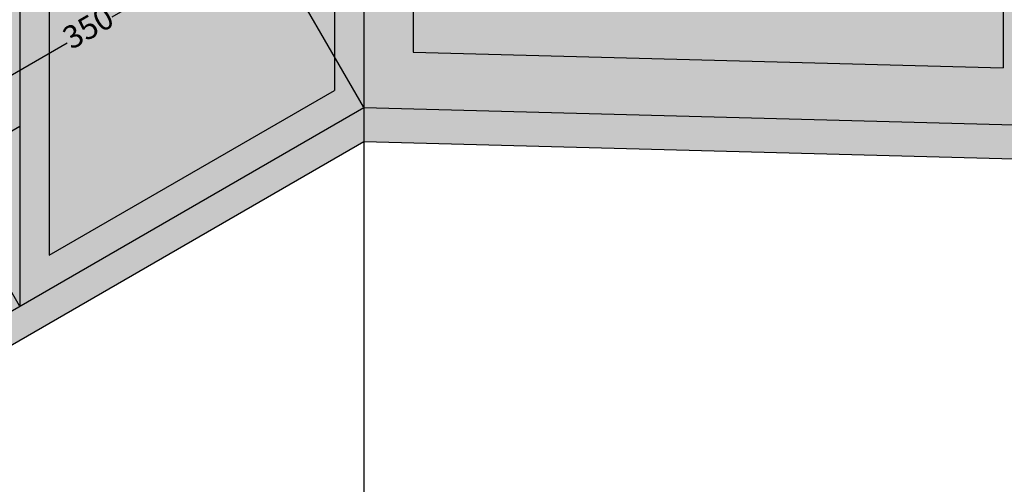
# Model space of a CAD drawing. Units: millimetres. Extents: x 78378 to 86415, y 148682 to 152721.
# Tile 7 of 18: x 79783 to 80650, y 149298 to 149707. Entities that reach past the tile are written whole.
import ezdxf

# ---------------------------------------------------------------- set-up
doc = ezdxf.new("R2010")
doc.units = ezdxf.units.MM
for name, color, linetype, lineweight in [('A-ANNO-DIMS', 2, 'Continuous', 18), ('A-FURN', 4, 'Continuous', 25), ('A-FURN-PATT', 32, 'Continuous', 13)]:
    doc.layers.add(name, color=color, linetype=linetype, lineweight=lineweight)
doc.styles.get("Standard").update_dxf_attribs({"font": 'arial.ttf'})
doc.dimstyles.new('ISO-25', dxfattribs={"dimtxt": 20, "dimasz": 20, "dimexe": 1.25, "dimexo": 0.625, "dimtad": 0, "dimdec": 1, "dimtxsty": 'Standard', "dimcen": 2.5, "dimadec": 0, "dimazin": 0, "dimtfac": 1, "dimtdec": 1, "dimtmove": 0, "dimatfit": 3, "dimfxl": 1, "dimarcsym": 0})

# ---------------------------------------------------------------- blocks, each defined once
blk = doc.blocks.new('*D22')
at = {"layer": 'A-ANNO-DIMS', "color": 0, "lineweight": -2, "transparency": 16777216}
for p, q in [((80086.09, 149630.55), (79995.78, 149786.97)), ((79979.08, 149775.89), (79864.49, 149709.73)), ((79710.62, 149620.89), (79825.21, 149687.05)), ((79782.98, 149455.55), (79692.67, 149611.97))]:
    blk.add_line(p, q, dxfattribs=at)
at = {"layer": 'A-ANNO-DIMS', "color": 0, "transparency": 16777216}
for points in [[(79977.42, 149778.78), (79980.75, 149773.01), (79996.4, 149785.89)], [(79708.95, 149623.78), (79712.28, 149618.01), (79693.3, 149610.89)]]:
    blk.add_solid(points, dxfattribs=at)
at = {"layer": 'Defpoints', "color": 0, "transparency": 16777216}
for p in [(79996.4, 149785.89), (80086.4, 149630.01), (79783.3, 149455.01)]:
    blk.add_point(p, dxfattribs=at)
at = {"layer": 'A-ANNO-DIMS', "color": 0, "transparency": 16777216, "insert": (79844.85, 149698.39), "char_height": 20, "attachment_point": 5, "rotation": 30}
blk.add_mtext('350', dxfattribs=at)
blk = doc.blocks.new('*D32')
at = {"layer": 'A-ANNO-DIMS', "color": 0, "lineweight": -2, "transparency": 16777216}
for p, q in [((80086.4, 150459.38), (80086.4, 148693.76)), ((80692.62, 150459.38), (80692.62, 148693.76)), ((80106.4, 148695.01), (80355.19, 148695.01)), ((80672.62, 148695.01), (80423.84, 148695.01))]:
    blk.add_line(p, q, dxfattribs=at)
at = {"layer": 'A-ANNO-DIMS', "color": 0, "transparency": 16777216}
for points in [[(80106.4, 148698.34), (80106.4, 148691.67), (80086.4, 148695.01)], [(80672.62, 148698.34), (80672.62, 148691.67), (80692.62, 148695.01)]]:
    blk.add_solid(points, dxfattribs=at)
at = {"layer": 'Defpoints', "color": 0, "transparency": 16777216}
for p in [(80086.4, 150460.01), (80692.62, 150460.01), (80692.62, 148695.01)]:
    blk.add_point(p, dxfattribs=at)
at = {"layer": 'A-ANNO-DIMS', "color": 0, "transparency": 16777216, "insert": (80389.51, 148695.01), "char_height": 20, "attachment_point": 5}
blk.add_mtext('606.2', dxfattribs=at)

msp = doc.modelspace()

# ---------------------------------------------------------------- hatches: boundary and pattern name
at = {"layer": 'A-FURN-PATT'}
h = msp.add_hatch(color=256, dxfattribs=at)
h.dxf.hatch_style = 1
h.paths.add_polyline_path([(80692.622, 150440.0076), (80086.4042, 150440.0076), (80086.4042, 149630.0076), (80692.622, 149614.0076)])
h.paths.add_polyline_path([(80293.421, 150335.1041, -0.69391375), (80505.0284, 150344.716, -0.266338), (80649.3207, 150178.1039), (80649.3207, 149665.1505), (80129.7055, 149678.8648), (80129.7055, 150178.1039, -0.25732621)], flags=16)
h.paths.add_polyline_path([(80060.4234, 150384.3024), (79809.2761, 150239.3024), (79809.2761, 150141.6366), (80060.4234, 150286.6366)])
h.paths.add_polyline_path([(80086.4042, 150399.3024), (80086.4042, 150440.0076), (79783.2953, 150265.0076), (79783.2953, 150224.3024)])
edge = h.paths.add_edge_path(flags=16)
edge.add_arc((79946.6302, 150348.8763), 10.7636, -18.3817969, 28.0331994, ccw=False)
edge.add_spline(control_points=[(79956.8447, 150345.482), (79949.4862, 150336.2391), (79933.8528, 150316.6023), (79908.9507, 150312.562), (79895.7699, 150310.4234)], knot_values=[0, 0, 0, 0, 34.22568399, 72.71357657, 72.71357657, 72.71357657, 72.71357657], degree=3, periodic=0)
edge.add_arc((79899.3869, 150314.0155), 5.0977, 123.6496153, 224.8024751, ccw=False)
edge.add_spline(control_points=[(79896.5622, 150318.259), (79909.861, 150320.2803), (79934.7821, 150324.0679), (79949.3412, 150344.4361), (79956.131, 150353.935)], knot_values=[0, 0, 0, 0, 38.48789258, 72.12331911, 72.12331911, 72.12331911, 72.12331911], degree=3, periodic=0)
h.paths.add_polyline_path([(80086.4042, 150399.3024), (80060.4234, 150384.3024), (80060.4234, 150286.6366), (80086.4042, 150301.6366)], flags=17)
h.paths.add_polyline_path([(79809.2761, 150239.3024), (79783.2953, 150224.3024), (79783.2953, 150126.6366), (79809.2761, 150141.6366)])
h = msp.add_hatch(color=256, dxfattribs=at)
h.dxf.hatch_style = 1
h.paths.add_polyline_path([(80060.4234, 150256.6366), (79809.2761, 150111.6366), (79809.2761, 149835.8221), (80060.4234, 149980.8221)])
edge = h.paths.add_edge_path(flags=16)
edge.add_arc((79897.9874, 150103.5556), 5.1726, 122.0794663, 231.0916039, ccw=False)
edge.add_spline(control_points=[(79895.2403, 150107.9384), (79905.0476, 150110.9384), (79924.6357, 150116.9304), (79948.7961, 150128.9973), (79958.1258, 150141.8088), (79961.3514, 150146.2382)], knot_values=[0, 0, 0, 0, 30.92804237, 61.77253951, 78.07166049, 78.07166049, 78.07166049, 78.07166049], degree=3, periodic=0)
edge.add_arc((79956.2102, 150141.1519), 7.232, -40.6762437, 44.6926573, ccw=False)
edge.add_spline(control_points=[(79961.695, 150136.4382), (79958.1075, 150132.5465), (79947.5299, 150121.0716), (79924.3289, 150108.3481), (79904.611, 150102.4724), (79894.7387, 150099.5306)], knot_values=[0, 0, 0, 0, 15.82960645, 46.67410358, 77.60214595, 77.60214595, 77.60214595, 77.60214595], degree=3, periodic=0)
h.paths.add_polyline_path([(80060.4234, 149950.8221), (79809.2761, 149805.8221), (79809.2761, 149500.0076), (80060.4234, 149645.0076)])
h.paths.add_polyline_path([(80649.3207, 150178.1039, 0.266338), (80505.0284, 150344.716, 0.69391375), (80293.421, 150335.1041, 0.25732621), (80129.7055, 150178.1039), (80129.7055, 149678.8648), (80649.3207, 149665.1505)])
h = msp.add_hatch(color=256, dxfattribs=at)
h.dxf.hatch_style = 1
h.paths.add_polyline_path([(79765.9748, 149445.0076), (79765.9748, 149603.6184), (79275.1761, 149320.2556), (79275.1761, 149161.6449), (79350.2826, 149205.0076)])
edge = h.paths.add_edge_path(flags=16)
edge.add_arc((79507.244, 149406.7325), 51.4573, 189.4892034, 208.9818028, ccw=False)
edge.add_spline(control_points=[(79456.4908, 149398.2492), (79490.7805, 149406.8496), (79544.6682, 149420.3656), (79585.6167, 149461.099), (79597.2078, 149478.6257), (79597.8866, 149479.6521)], knot_values=[0, 0, 0, 0, 103.87115175, 163.23805465, 166.93094527, 166.93094527, 166.93094527, 166.93094527], degree=3, periodic=0)
edge.add_arc((79598.468, 149470.6289), 9.0419, -55.2157026, 93.6867088, ccw=False)
edge.add_spline(control_points=[(79603.6263, 149463.2027), (79602.9475, 149462.1763), (79591.3564, 149444.6496), (79550.4079, 149403.9163), (79496.5202, 149390.4003), (79462.2305, 149381.7998)], knot_values=[0, 0, 0, 0, 3.69289062, 63.05979352, 166.93094527, 166.93094527, 166.93094527, 166.93094527], degree=3, periodic=0)
h.paths.add_polyline_path([(80060.4234, 149980.8221), (80060.4234, 150256.6366), (79809.2761, 150111.6366), (79809.2761, 149835.8221)], flags=0)
edge = h.paths.add_edge_path(flags=0)
edge.add_arc((79897.9874, 150103.5556), 5.1726, 122.0794663, 231.0916039, ccw=False)
edge.add_spline(control_points=[(79895.2403, 150107.9384), (79905.0476, 150110.9384), (79924.6357, 150116.9304), (79948.7961, 150128.9973), (79958.1258, 150141.8088), (79961.3514, 150146.2382)], knot_values=[0, 0, 0, 0, 30.92804237, 61.77253951, 78.07166049, 78.07166049, 78.07166049, 78.07166049], degree=3, periodic=0)
edge.add_arc((79956.2102, 150141.1519), 7.232, -40.6762437, 44.6926573, ccw=False)
edge.add_spline(control_points=[(79961.695, 150136.4382), (79958.1075, 150132.5465), (79947.5299, 150121.0716), (79924.3289, 150108.3481), (79904.611, 150102.4724), (79894.7387, 150099.5306)], knot_values=[0, 0, 0, 0, 15.82960645, 46.67410358, 77.60214595, 77.60214595, 77.60214595, 77.60214595], degree=3, periodic=0)
h.paths.add_polyline_path([(80060.4234, 149950.8221), (79809.2761, 149805.8221), (79809.2761, 149500.0076), (80060.4234, 149645.0076)], flags=0)
edge = h.paths.add_edge_path(flags=0)
edge.add_arc((79897.9874, 149795.6302), 5.1726, 122.0794663, 231.0916039, ccw=False)
edge.add_spline(control_points=[(79895.2403, 149800.013), (79905.0476, 149803.013), (79924.6357, 149809.005), (79948.7961, 149821.0719), (79958.1258, 149833.8834), (79961.3514, 149838.3128)], knot_values=[0, 0, 0, 0, 30.92804237, 61.77253951, 78.07166049, 78.07166049, 78.07166049, 78.07166049], degree=3, periodic=0)
edge.add_arc((79956.2102, 149833.2265), 7.232, -40.6762437, 44.6926573, ccw=False)
edge.add_spline(control_points=[(79961.695, 149828.5129), (79958.1075, 149824.6211), (79947.5299, 149813.1462), (79924.3289, 149800.4227), (79904.611, 149794.547), (79894.7387, 149791.6052)], knot_values=[0, 0, 0, 0, 15.82960645, 46.67410358, 77.60214595, 77.60214595, 77.60214595, 77.60214595], degree=3, periodic=0)
h.paths.add_polyline_path([(80086.4042, 150301.6366), (79783.2953, 150126.6366), (79783.2953, 149455.0076), (80086.4042, 149630.0076)])
h.paths.add_polyline_path([(79809.2761, 150111.6366), (80060.4234, 150256.6366), (80060.4234, 149980.8221), (79809.2761, 149835.8221)], flags=16)
h.paths.add_polyline_path([(80060.4234, 149950.8221), (80060.4234, 149645.0076), (79809.2761, 149500.0076), (79809.2761, 149805.8221)], flags=16)
h = msp.add_hatch(color=256, dxfattribs=at)
h.dxf.hatch_style = 1
h.paths.add_polyline_path([(79765.9748, 150214.3024), (79275.1761, 149930.9396), (79275.1761, 149340.2556), (79361.1019, 149389.8649), (79361.1019, 149854.0252), (79688.5392, 150043.0712), (79688.5392, 149578.9109), (79765.9748, 149623.6184)], flags=0)
h.paths.add_polyline_path([(79616.9975, 150064.3358, -1), (79579.5778, 150064.3358, -1)], flags=0)
h.paths.add_polyline_path([(79511.257, 150003.2865, -1), (79473.8373, 150003.2865, -1)], flags=0)
h.paths.add_polyline_path([(79398.6146, 149938.2524, -1), (79361.1949, 149938.2524, -1)], flags=0)
h.paths.add_polyline_path([(79688.5392, 149578.9109), (79667.1607, 149674.8368), (79401.2524, 149521.3146), (79361.1019, 149389.8649)], flags=0)
h.paths.add_polyline_path([(79783.2953, 149613.6184), (79783.2953, 150126.6366), (79783.2953, 150265.0076), (79257.8556, 149961.6449), (79257.8556, 149310.2556)])
h.paths.add_polyline_path([(79275.1761, 149340.2556), (79275.1761, 149930.9396), (79765.9748, 150214.3024), (79765.9748, 149623.6184)], flags=16)
h.paths.add_polyline_path([(79361.1019, 149389.8649), (79361.1019, 149854.0252), (79688.5392, 150043.0712), (79688.5392, 149578.9109), (79667.1607, 149674.8368), (79401.2524, 149521.3146)], flags=0)
h.paths.add_polyline_path([(79477.9029, 149864.6773), (79477.9029, 149877.6076), (79571.7852, 149931.8105), (79571.7852, 149918.8803)], flags=0)
h = msp.add_hatch(color=256, dxfattribs=at)
h.dxf.hatch_style = 1
h.paths.add_polyline_path([(81125.6347, 150190.0076), (81116.9744, 150195.0076), (81116.9744, 149762.4135), (81125.6347, 149757.4135)])
h.paths.add_polyline_path([(81125.6347, 149757.4135), (81116.9744, 149762.4135), (81116.9744, 149732.4135), (81125.6347, 149727.4135)])
h.paths.add_polyline_path([(79275.1761, 149320.2556), (79257.8556, 149310.2556), (79257.8556, 149151.6449), (79275.1761, 149161.6449)])
h.paths.add_polyline_path([(79783.2953, 149613.6184), (79765.9748, 149603.6184), (79765.9748, 149445.0076), (79783.2953, 149455.0076)])
h.paths.add_polyline_path([(79765.9748, 149445.0076), (79765.9748, 149603.6184), (79275.1761, 149320.2556), (79275.1761, 149161.6449), (79350.2826, 149205.0076)])
edge = h.paths.add_edge_path(flags=0)
edge.add_spline(control_points=[(79456.4908, 149398.2492), (79490.7805, 149406.8496), (79544.6682, 149420.3656), (79585.6167, 149461.099), (79597.2078, 149478.6257), (79597.8866, 149479.6521)], knot_values=[0, 0, 0, 0, 103.87115175, 163.23805465, 166.93094527, 166.93094527, 166.93094527, 166.93094527], degree=3, periodic=0)
edge.add_arc((79598.468, 149470.6289), 9.0419, -55.2157026, 93.6867088, ccw=False)
edge.add_spline(control_points=[(79603.6263, 149463.2027), (79602.9475, 149462.1763), (79591.3564, 149444.6496), (79550.4079, 149403.9163), (79496.5202, 149390.4003), (79462.2305, 149381.7998)], knot_values=[0, 0, 0, 0, 3.69289062, 63.05979352, 166.93094527, 166.93094527, 166.93094527, 166.93094527], degree=3, periodic=0)
edge.add_arc((79507.244, 149406.7325), 51.4573, 189.4892034, 208.9818028, ccw=False)
edge = h.paths.add_edge_path(flags=16)
edge.add_spline(control_points=[(79462.2305, 149381.7998), (79496.5202, 149390.4003), (79550.4079, 149403.9163), (79591.3564, 149444.6496), (79602.9475, 149462.1763), (79603.6263, 149463.2027)], knot_values=[0, 0, 0, 0, 103.87115175, 163.23805465, 166.93094527, 166.93094527, 166.93094527, 166.93094527], degree=3, periodic=0)
edge.add_arc((79598.468, 149470.6289), 9.0419, 304.7842974, 453.6867088)
edge.add_spline(control_points=[(79597.8866, 149479.6521), (79597.2078, 149478.6257), (79585.6167, 149461.099), (79544.6682, 149420.3656), (79490.7805, 149406.8496), (79456.4908, 149398.2492)], knot_values=[0, 0, 0, 0, 3.69289062, 63.05979352, 166.93094527, 166.93094527, 166.93094527, 166.93094527], degree=3, periodic=0)
edge.add_arc((79507.244, 149406.7325), 51.4573, 189.4892034, 208.9818028)
h = msp.add_hatch(color=256, dxfattribs=at)
h.dxf.hatch_style = 1
h.paths.add_polyline_path([(80086.4042, 149600.0076), (80692.622, 149584.0076), (81239.9694, 149267.9965), (81239.9694, 149297.9965), (81116.9744, 149369.0076), (80692.622, 149614.0076), (80086.4042, 149630.0076), (78830.6674, 148905.0076), (78830.6674, 148875.0076)])

# ---------------------------------------------------------------- linework, layer by layer
at = {"layer": 'A-FURN'}
for p, q in [((80086.4042, 150460.0076), (80086.4042, 149630.0076)), ((79783.2953, 150285.0076), (79783.2953, 149455.0076)), ((80129.7055, 150178.1039), (80129.7055, 149678.8648)), ((80649.3207, 150178.1039), (80649.3207, 149665.1505)), ((79783.2953, 150126.6366), (79783.2953, 149455.0076)), ((80060.4234, 149950.8221), (80060.4234, 149645.0076)), ((79809.2761, 149805.8221), (79809.2761, 149500.0076)), ((80129.7055, 149678.8648), (80649.3207, 149665.1505)), ((79809.2761, 149500.0076), (80060.4234, 149645.0076)), ((78830.6674, 148905.0076), (80086.4042, 149630.0076)), ((80086.4042, 149630.0076), (80692.622, 149614.0076)), ((79257.8556, 149310.2556), (79783.2953, 149613.6184)), ((78830.6674, 148875.0076), (80086.4042, 149600.0076)), ((80086.4042, 149600.0076), (80692.622, 149584.0076))]:
    msp.add_line(p, q, dxfattribs=at)

# ---------------------------------------------------------------- dimensions: what is measured, and where the dimension line sits
at = {"layer": 'A-ANNO-DIMS'}
dim = msp.add_linear_dim(base=(80692.622, 148695.0076), p1=(80086.4042, 150460.0076), p2=(80692.622, 150460.0076), dimstyle='ISO-25', override={"dimdec": 1, "dimlfac": 1, "dimrnd": 0, "dimzin": 0, "dimdsep": 46, "dimlunit": 2}, dxfattribs=at)
dim.commit()
dim.dimension.update_dxf_attribs({"geometry": '*D32', "text_midpoint": (80389.5131, 148695.0076)})
dim = msp.add_linear_dim(base=(79996.4042, 149785.8922), p1=(79783.2953, 149455.0076), p2=(80086.4042, 149630.0076), angle=30, dimstyle='ISO-25', override={"dimdec": 0, "dimlfac": 1, "dimrnd": 0, "dimzin": 0, "dimdsep": 46, "dimlunit": 2}, dxfattribs=at)
dim.commit()
dim.dimension.update_dxf_attribs({"geometry": '*D22', "text_midpoint": (79844.8498, 149698.3922)})

doc.saveas('drawing.dxf')
